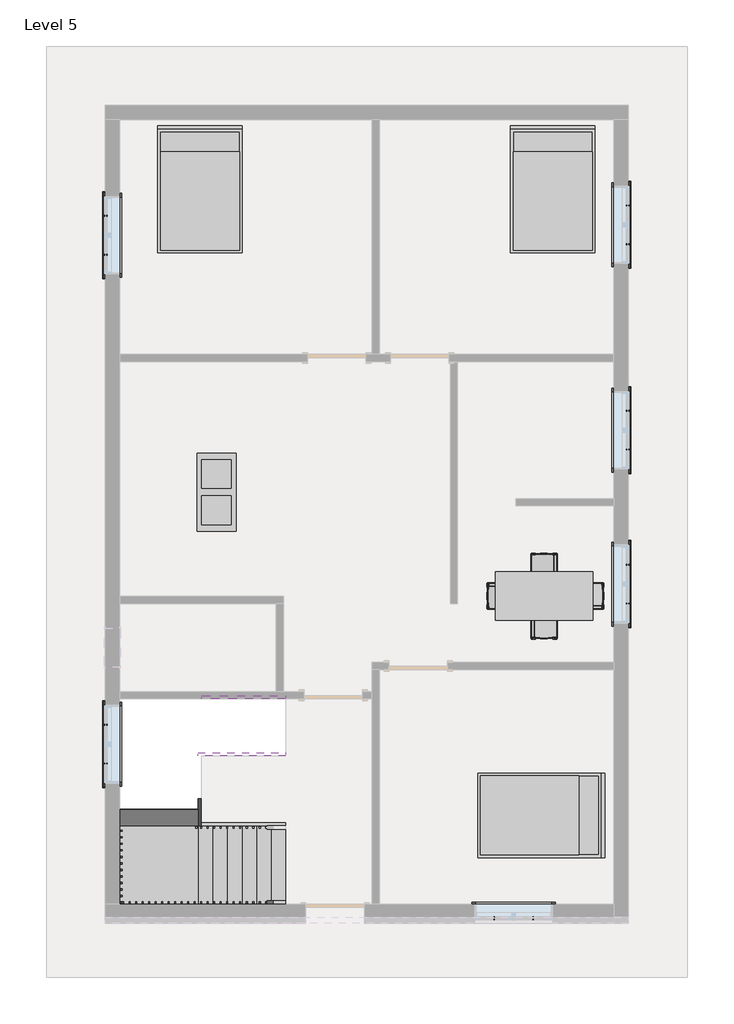
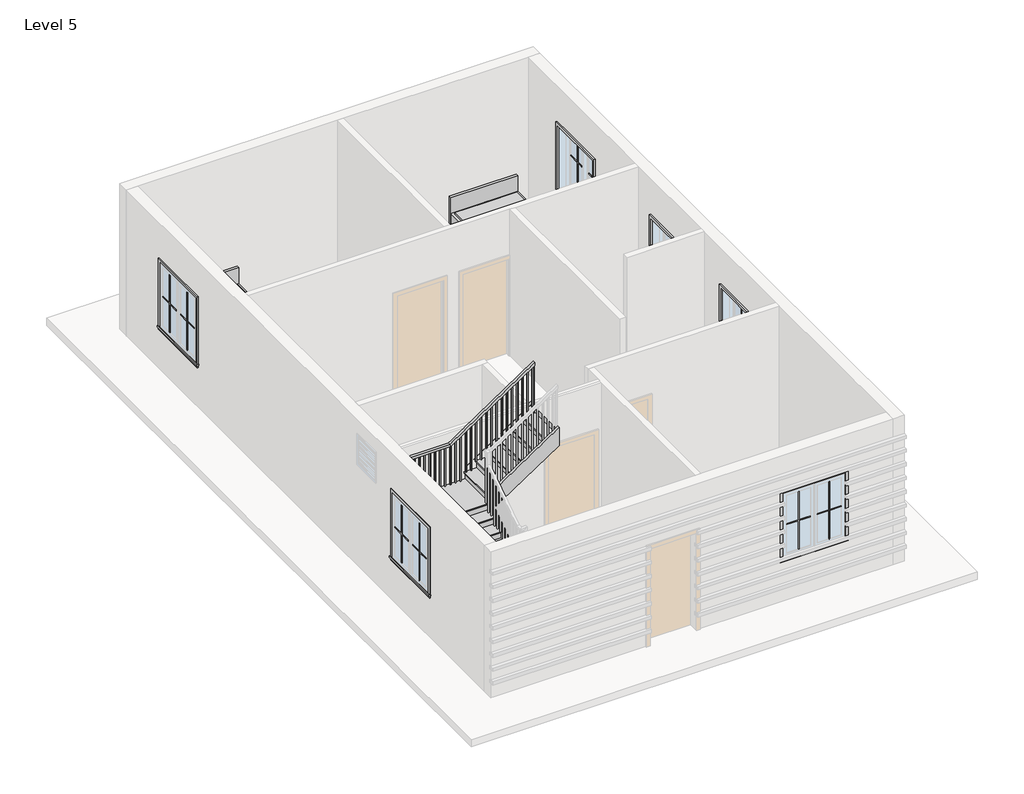
# One storey, part 3 of 3: 25 proxies, 5 members, 4 furniture elements, 1 railing, 1 stair flight.
"""IFC4 building model written with IfcOpenShell, lengths in millimetres."""

from ifc_helpers import new_model, si_unit, frame, origin, place, context, project, spatial, polyline, outline, extrude, faceted_brep, transform, mapped, element, save
from components import muntin_pattern_2x2_muntin_pattern_2x2_ba8901dc, muntin_pattern_2x2_muntin_pattern_2x2_877df4e9, trim_window_exterior_flat_with_sill_fda35bc9, trim_window_interior_flat_picture_frame_a80dbcd9, coffee_table_with_brass_mullions_11320_coffee_table_with_5962bef7, bed_17739_bed_17739_15c61121, dining_table_w_chairs_11374_0cdfc61b, stair_flight_e1114729

model = new_model("IFC4")

# Units and contexts
model_context = context("Model", 3, world=origin())
ifc_project = project(units=[si_unit("LENGTHUNIT", "METRE", prefix="MILLI")], contexts=[model_context])

# Site, building, storey
site = spatial("IfcSite", under=ifc_project)
building = spatial("IfcBuilding", under=site)
storey = spatial("IfcBuildingStorey", under=building, Name="Level 5", Elevation=12649.2)

# Proxies
placement = place(None, origin())
muntin_pattern_2x2_muntin_pattern_2x2_shape = muntin_pattern_2x2_muntin_pattern_2x2_ba8901dc(model_context)
element("IfcBuildingElementProxy", 1, Name="Muntin Pattern_2x2 : Muntin Pattern_2x2", ObjectType="Muntin Pattern_2x2 : Muntin Pattern_2x2", at=placement, inside=storey, context=model_context, shape_type="MappedRepresentation", body=[
    mapped(muntin_pattern_2x2_muntin_pattern_2x2_shape, transform((-5325.0867403, -4189.9051559, 13633.45), x_axis=(0.0, 1.0, 0.0), y_axis=(-1.0, 0.0, 0.0), z_axis=(0.0, 0.0, 1.0))),
])
element("IfcBuildingElementProxy", 2, Name="Muntin Pattern_2x2 : Muntin Pattern_2x2", ObjectType="Muntin Pattern_2x2 : Muntin Pattern_2x2", at=placement, inside=storey, context=model_context, shape_type="MappedRepresentation", body=[
    mapped(muntin_pattern_2x2_muntin_pattern_2x2_shape, transform((-5325.0867403, 3744.4198441, 13633.45), x_axis=(0.0, 1.0, 0.0), y_axis=(-1.0, 0.0, 0.0), z_axis=(0.0, 0.0, 1.0))),
])
element("IfcBuildingElementProxy", 3, Name="Muntin Pattern_2x2 : Muntin Pattern_2x2", ObjectType="Muntin Pattern_2x2 : Muntin Pattern_2x2", at=placement, inside=storey, context=model_context, shape_type="MappedRepresentation", body=[
    mapped(muntin_pattern_2x2_muntin_pattern_2x2_shape, transform((2821.9632597, 4512.7698441, 13633.45), x_axis=(0.0, -1.0, 0.0), y_axis=(1.0, 0.0, 0.0), z_axis=(0.0, 0.0, 1.0))),
])
element("IfcBuildingElementProxy", 4, Name="Muntin Pattern_2x2 : Muntin Pattern_2x2", ObjectType="Muntin Pattern_2x2 : Muntin Pattern_2x2", at=placement, inside=storey, context=model_context, shape_type="MappedRepresentation", body=[
    mapped(muntin_pattern_2x2_muntin_pattern_2x2_shape, transform((2821.9632597, 1312.3698441, 13633.45), x_axis=(0.0, -1.0, 0.0), y_axis=(1.0, 0.0, 0.0), z_axis=(0.0, 0.0, 1.0))),
])
element("IfcBuildingElementProxy", 5, Name="Muntin Pattern_2x2 : Muntin Pattern_2x2", ObjectType="Muntin Pattern_2x2 : Muntin Pattern_2x2", at=placement, inside=storey, context=model_context, shape_type="MappedRepresentation", body=[
    mapped(muntin_pattern_2x2_muntin_pattern_2x2_shape, transform((2821.9632597, -1087.9301559, 13633.45), x_axis=(0.0, -1.0, 0.0), y_axis=(1.0, 0.0, 0.0), z_axis=(0.0, 0.0, 1.0))),
])
element("IfcBuildingElementProxy", 6, Name="Muntin Pattern_2x2 : Muntin Pattern_2x2", ObjectType="Muntin Pattern_2x2 : Muntin Pattern_2x2", at=placement, inside=storey, context=model_context, shape_type="MappedRepresentation", body=[
    mapped(muntin_pattern_2x2_muntin_pattern_2x2_shape, transform((1344.0007597, -6601.3176559, 13633.45), x_axis=(-1.0, 0.0, 0.0), y_axis=(0.0, -1.0, 0.0), z_axis=(0.0, 0.0, 1.0))),
])
muntin_pattern_2x2_muntin_pattern_2x2_2_shape = muntin_pattern_2x2_muntin_pattern_2x2_877df4e9(model_context)
element("IfcBuildingElementProxy", 7, Name="Muntin Pattern_2x2 : Muntin Pattern_2x2", ObjectType="Muntin Pattern_2x2 : Muntin Pattern_2x2", at=placement, inside=storey, context=model_context, shape_type="MappedRepresentation", body=[
    mapped(muntin_pattern_2x2_muntin_pattern_2x2_2_shape, transform((-5325.0867403, -3583.4801559, 13633.45), x_axis=(0.0, -1.0, 0.0), y_axis=(1.0, 0.0, 0.0), z_axis=(0.0, 0.0, 1.0))),
])
element("IfcBuildingElementProxy", 8, Name="Muntin Pattern_2x2 : Muntin Pattern_2x2", ObjectType="Muntin Pattern_2x2 : Muntin Pattern_2x2", at=placement, inside=storey, context=model_context, shape_type="MappedRepresentation", body=[
    mapped(muntin_pattern_2x2_muntin_pattern_2x2_2_shape, transform((-5325.0867403, 4350.8448441, 13633.45), x_axis=(0.0, -1.0, 0.0), y_axis=(1.0, 0.0, 0.0), z_axis=(0.0, 0.0, 1.0))),
])
element("IfcBuildingElementProxy", 9, Name="Muntin Pattern_2x2 : Muntin Pattern_2x2", ObjectType="Muntin Pattern_2x2 : Muntin Pattern_2x2", at=placement, inside=storey, context=model_context, shape_type="MappedRepresentation", body=[
    mapped(muntin_pattern_2x2_muntin_pattern_2x2_2_shape, transform((2821.9632597, 3906.3448441, 13633.45), x_axis=(0.0, 1.0, 0.0), y_axis=(-1.0, 0.0, 0.0), z_axis=(0.0, 0.0, 1.0))),
])
element("IfcBuildingElementProxy", 10, Name="Muntin Pattern_2x2 : Muntin Pattern_2x2", ObjectType="Muntin Pattern_2x2 : Muntin Pattern_2x2", at=placement, inside=storey, context=model_context, shape_type="MappedRepresentation", body=[
    mapped(muntin_pattern_2x2_muntin_pattern_2x2_2_shape, transform((2821.9632597, 705.9448441, 13633.45), x_axis=(0.0, 1.0, 0.0), y_axis=(-1.0, 0.0, 0.0), z_axis=(0.0, 0.0, 1.0))),
])
element("IfcBuildingElementProxy", 11, Name="Muntin Pattern_2x2 : Muntin Pattern_2x2", ObjectType="Muntin Pattern_2x2 : Muntin Pattern_2x2", at=placement, inside=storey, context=model_context, shape_type="MappedRepresentation", body=[
    mapped(muntin_pattern_2x2_muntin_pattern_2x2_2_shape, transform((2821.9632597, -1694.3551559, 13633.45), x_axis=(0.0, 1.0, 0.0), y_axis=(-1.0, 0.0, 0.0), z_axis=(0.0, 0.0, 1.0))),
])
element("IfcBuildingElementProxy", 12, Name="Muntin Pattern_2x2 : Muntin Pattern_2x2", ObjectType="Muntin Pattern_2x2 : Muntin Pattern_2x2", at=placement, inside=storey, context=model_context, shape_type="MappedRepresentation", body=[
    mapped(muntin_pattern_2x2_muntin_pattern_2x2_2_shape, transform((737.5757597, -6601.3176559, 13633.45), x_axis=(1.0, 0.0, 0.0), y_axis=(0.0, 1.0, 0.0), z_axis=(0.0, 0.0, 1.0))),
])
trim_window_exterior_flat_with_sill_shape = trim_window_exterior_flat_with_sill_fda35bc9(model_context)
element("IfcBuildingElementProxy", 13, Name="Trim-Window-Exterior-Flat : with Sill", ObjectType="Trim-Window-Exterior-Flat : with Sill", at=placement, inside=storey, context=model_context, shape_type="MappedRepresentation", body=[
    mapped(trim_window_exterior_flat_with_sill_shape, transform((-5334.6117403, -3886.6926559, 14909.8), x_axis=(0.0, -1.0, 0.0), y_axis=(0.0, 0.0, 1.0), z_axis=(-1.0, 0.0, 0.0))),
])
element("IfcBuildingElementProxy", 14, Name="Trim-Window-Exterior-Flat : with Sill", ObjectType="Trim-Window-Exterior-Flat : with Sill", at=placement, inside=storey, context=model_context, shape_type="MappedRepresentation", body=[
    mapped(trim_window_exterior_flat_with_sill_shape, transform((-5334.6117403, 4047.6323441, 14909.8), x_axis=(0.0, -1.0, 0.0), y_axis=(0.0, 0.0, 1.0), z_axis=(-1.0, 0.0, 0.0))),
])
element("IfcBuildingElementProxy", 15, Name="Trim-Window-Exterior-Flat : with Sill", ObjectType="Trim-Window-Exterior-Flat : with Sill", at=placement, inside=storey, context=model_context, shape_type="MappedRepresentation", body=[
    mapped(trim_window_exterior_flat_with_sill_shape, transform((2831.4882597, 4209.5573441, 14909.8), x_axis=(0.0, 1.0, 0.0), y_axis=(0.0, 0.0, 1.0), z_axis=(1.0, 0.0, 0.0))),
])
element("IfcBuildingElementProxy", 16, Name="Trim-Window-Exterior-Flat : with Sill", ObjectType="Trim-Window-Exterior-Flat : with Sill", at=placement, inside=storey, context=model_context, shape_type="MappedRepresentation", body=[
    mapped(trim_window_exterior_flat_with_sill_shape, transform((2831.4882597, 1009.1573441, 14909.8), x_axis=(0.0, 1.0, 0.0), y_axis=(0.0, 0.0, 1.0), z_axis=(1.0, 0.0, 0.0))),
])
element("IfcBuildingElementProxy", 17, Name="Trim-Window-Exterior-Flat : with Sill", ObjectType="Trim-Window-Exterior-Flat : with Sill", at=placement, inside=storey, context=model_context, shape_type="MappedRepresentation", body=[
    mapped(trim_window_exterior_flat_with_sill_shape, transform((2831.4882597, -1391.1426559, 14909.8), x_axis=(0.0, 1.0, 0.0), y_axis=(0.0, 0.0, 1.0), z_axis=(1.0, 0.0, 0.0))),
])
element("IfcBuildingElementProxy", 18, Name="Trim-Window-Exterior-Flat : with Sill", ObjectType="Trim-Window-Exterior-Flat : with Sill", at=placement, inside=storey, context=model_context, shape_type="MappedRepresentation", body=[
    mapped(trim_window_exterior_flat_with_sill_shape, transform((1040.7882597, -6610.8426559, 14909.8), x_axis=(1.0, 0.0, 0.0), y_axis=(0.0, 0.0, 1.0), z_axis=(0.0, -1.0, 0.0))),
])
trim_window_interior_flat_picture_frame_shape = trim_window_interior_flat_picture_frame_a80dbcd9(model_context)
element("IfcBuildingElementProxy", 19, Name="Trim-Window-Interior-Flat : Picture Frame", ObjectType="Trim-Window-Interior-Flat : Picture Frame", at=placement, inside=storey, context=model_context, shape_type="MappedRepresentation", body=[
    mapped(trim_window_interior_flat_picture_frame_shape, transform((-5106.0117403, -3886.6926559, 14909.8), x_axis=(0.0, 1.0, 0.0), y_axis=(0.0, 0.0, 1.0), z_axis=(1.0, 0.0, 0.0))),
])
element("IfcBuildingElementProxy", 20, Name="Trim-Window-Interior-Flat : Picture Frame", ObjectType="Trim-Window-Interior-Flat : Picture Frame", at=placement, inside=storey, context=model_context, shape_type="MappedRepresentation", body=[
    mapped(trim_window_interior_flat_picture_frame_shape, transform((-5106.0117403, 4047.6323441, 14909.8), x_axis=(0.0, 1.0, 0.0), y_axis=(0.0, 0.0, 1.0), z_axis=(1.0, 0.0, 0.0))),
])
element("IfcBuildingElementProxy", 21, Name="Trim-Window-Interior-Flat : Picture Frame", ObjectType="Trim-Window-Interior-Flat : Picture Frame", at=placement, inside=storey, context=model_context, shape_type="MappedRepresentation", body=[
    mapped(trim_window_interior_flat_picture_frame_shape, transform((2602.8882597, 4209.5573441, 14909.8), x_axis=(0.0, -1.0, 0.0), y_axis=(0.0, 0.0, 1.0), z_axis=(-1.0, 0.0, 0.0))),
])
element("IfcBuildingElementProxy", 22, Name="Trim-Window-Interior-Flat : Picture Frame", ObjectType="Trim-Window-Interior-Flat : Picture Frame", at=placement, inside=storey, context=model_context, shape_type="MappedRepresentation", body=[
    mapped(trim_window_interior_flat_picture_frame_shape, transform((2602.8882597, 1009.1573441, 14909.8), x_axis=(0.0, -1.0, 0.0), y_axis=(0.0, 0.0, 1.0), z_axis=(-1.0, 0.0, 0.0))),
])
element("IfcBuildingElementProxy", 23, Name="Trim-Window-Interior-Flat : Picture Frame", ObjectType="Trim-Window-Interior-Flat : Picture Frame", at=placement, inside=storey, context=model_context, shape_type="MappedRepresentation", body=[
    mapped(trim_window_interior_flat_picture_frame_shape, transform((2602.8882597, -1391.1426559, 14909.8), x_axis=(0.0, -1.0, 0.0), y_axis=(0.0, 0.0, 1.0), z_axis=(-1.0, 0.0, 0.0))),
])
element("IfcBuildingElementProxy", 24, Name="Trim-Window-Interior-Flat : Picture Frame", ObjectType="Trim-Window-Interior-Flat : Picture Frame", at=placement, inside=storey, context=model_context, shape_type="MappedRepresentation", body=[
    mapped(trim_window_interior_flat_picture_frame_shape, transform((1040.7882597, -6382.2426559, 14909.8), x_axis=(-1.0, 0.0, 0.0), y_axis=(0.0, 0.0, 1.0), z_axis=(0.0, 1.0, 0.0))),
])
coffee_table_with_brass_mullions_11320_coffee_table_with_shape = coffee_table_with_brass_mullions_11320_coffee_table_with_5962bef7(model_context)
element("IfcBuildingElementProxy", 25, Name="coffee_table_with_brass_mullions_11320 : coffee_table_with_brass_mullions_11320", ObjectType="coffee_table_with_brass_mullions_11320 : coffee_table_with_brass_mullions_11320", at=placement, inside=storey, context=model_context, shape_type="MappedRepresentation", body=[
    mapped(coffee_table_with_brass_mullions_11320_coffee_table_with_shape, transform((-3162.9117403, 678.9573441, 12649.2), x_axis=(0.0, 1.0, 0.0), y_axis=(-1.0, 0.0, 0.0), z_axis=(0.0, 0.0, 1.0))),
])

# Furniture
bed_17739_bed_17739_shape = bed_17739_bed_17739_15c61121(model_context)
element("IfcFurniture", 26, ObjectType="Bed_17739 : Bed_17739", at=placement, inside=storey, context=model_context, shape_type="MappedRepresentation", body=[
    mapped(bed_17739_bed_17739_shape, transform((-3855.0617403, 4742.9573441, 12649.2), x_axis=(1.0, 0.0, 0.0), y_axis=(0.0, 1.0, 0.0), z_axis=(0.0, 0.0, 1.0))),
])
element("IfcFurniture", 27, ObjectType="Bed_17739 : Bed_17739", at=placement, inside=storey, context=model_context, shape_type="MappedRepresentation", body=[
    mapped(bed_17739_bed_17739_shape, transform((1650.3882597, 4742.9573441, 12649.2), x_axis=(1.0, 0.0, 0.0), y_axis=(0.0, 1.0, 0.0), z_axis=(0.0, 0.0, 1.0))),
])
element("IfcFurniture", 28, ObjectType="Bed_17739 : Bed_17739", at=placement, inside=storey, context=model_context, shape_type="MappedRepresentation", body=[
    mapped(bed_17739_bed_17739_shape, transform((1447.1882597, -4997.9426559, 12649.2), x_axis=(0.0, -1.0, 0.0), y_axis=(1.0, 0.0, 0.0), z_axis=(0.0, 0.0, 1.0))),
])
dining_table_w_chairs_11374_shape = dining_table_w_chairs_11374_0cdfc61b(model_context)
element("IfcFurniture", 29, ObjectType="Dining_Table_w_Chairs_11374", at=placement, inside=storey, context=model_context, shape_type="MappedRepresentation", body=[
    mapped(dining_table_w_chairs_11374_shape, transform((1497.0410232, -1671.6886654, 12649.2), x_axis=(1.0, 0.0, 0.0), y_axis=(0.0, 1.0, 0.0), z_axis=(0.0, 0.0, 1.0))),
])

# Members
element("IfcMember", 30, ObjectType="Stringer - 2\" Width", at=placement, inside=storey, context=model_context, shape_type="SweptSolid", body=[
    extrude(outline(polyline([(12649.2, -2515.2117403), (12867.2398409, -2515.2117403), (13121.2398409, -2896.2117403), (13121.2398409, -3445.6977546), (12649.2, -2737.6379933), (12649.2, -2515.2117403)])), frame((0.0, -6433.0426559, 0.0), z_axis=(0.0, 1.0, 0.0), x_axis=(0.0, 0.0, 1.0)), (0.0, 0.0, 1.0), 50.8),
])
element("IfcMember", 31, ObjectType="Stringer - 2\" Width", at=placement, inside=storey, context=model_context, shape_type="SweptSolid", body=[
    extrude(outline(polyline([(14888.5158313, -3277.2117403), (15396.5158313, -2515.2117403), (15762.8398409, -2515.2117403), (14888.5158313, -3826.6977546), (14888.5158313, -3277.2117403)])), frame((0.0, -3181.8426559, 0.0), z_axis=(0.0, 1.0, 0.0), x_axis=(0.0, 0.0, 1.0)), (0.0, 0.0, 1.0), 50.8),
])
element("IfcMember", 32, ObjectType="Stringer - 2\" Width", at=placement, inside=storey, context=model_context, shape_type="SweptSolid", body=[
    extrude(outline(polyline([(12649.2, -2515.2117403), (12867.2398409, -2515.2117403), (13747.7731743, -3836.0117403), (13381.4491647, -3836.0117403), (12649.2, -2737.6379933), (12649.2, -2515.2117403)])), frame((0.0, -5163.0426559, 0.0), z_axis=(0.0, 1.0, 0.0), x_axis=(0.0, 0.0, 1.0)), (0.0, 0.0, 1.0), 50.8),
])
element("IfcMember", 33, ObjectType="Stringer - 2\" Width", at=placement, inside=storey, context=model_context, shape_type="SweptSolid", body=[
    extrude(outline(polyline([(-5163.0426559, 13567.7158313), (-5163.0426559, 13934.0398409), (-4070.8426559, 14662.1731743), (-4070.8426559, 14295.8491647), (-5163.0426559, 13567.7158313)])), frame((-3886.8117403, 0.0, 0.0), z_axis=(1.0, 0.0, 0.0), x_axis=(0.0, 1.0, 0.0)), (0.0, 0.0, 1.0), 50.8),
])
element("IfcMember", 34, ObjectType="Stringer - 2\" Width", at=placement, inside=storey, context=model_context, shape_type="SweptSolid", body=[
    extrude(outline(polyline([(14848.4398409, -3886.8117403), (14482.1158313, -3886.8117403), (15396.5158313, -2515.2117403), (15762.8398409, -2515.2117403), (14848.4398409, -3886.8117403)])), frame((0.0, -4070.8426559, 0.0), z_axis=(0.0, 1.0, 0.0), x_axis=(0.0, 0.0, 1.0)), (0.0, 0.0, 1.0), 50.8),
])

# Railing
element("IfcRailing", 35, ObjectType="Handrail - Rectangular", at=placement, inside=storey, context=model_context, shape_type="SolidModel", body=[
    faceted_brep([(-2515.2117403, -6382.2426559, 13716.0), (-2515.2117403, -6382.2426559, 13654.9459984), (-2515.2117403, -6331.4426559, 13654.9459984), (-2515.2117403, -6331.4426559, 13716.0), (-4001.1117403, -6382.2426559, 14706.6), (-4016.4927427, -6382.2426559, 14655.8), (-4016.4927427, -6331.4426559, 14655.8), (-4001.1117403, -6331.4426559, 14706.6), (-5106.0117403, -6382.2426559, 14706.6), (-5106.0117403, -6382.2426559, 14655.8), (-5055.2117403, -6331.4426559, 14655.8), (-5055.2117403, -6331.4426559, 14706.6), (-5106.0117403, -5277.3426559, 14706.6), (-5106.0117403, -5261.9616535, 14655.8), (-5055.2117403, -5261.9616535, 14655.8), (-5055.2117403, -5277.3426559, 14706.6), (-5106.0117403, -4096.2426559, 15494.0), (-5106.0117403, -4080.8616535, 15443.2), (-5055.2117403, -4080.8616535, 15443.2), (-5055.2117403, -4096.2426559, 15494.0), (-5106.0117403, -3181.8426559, 15494.0), (-5106.0117403, -3181.8426559, 15443.2), (-5055.2117403, -3232.6426559, 15443.2), (-5055.2117403, -3232.6426559, 15494.0), (-4191.6117403, -3181.8426559, 15494.0), (-4176.2307379, -3181.8426559, 15443.2), (-4176.2307379, -3232.6426559, 15443.2), (-4191.6117403, -3232.6426559, 15494.0), (-2515.2117403, -3181.8426559, 16611.6), (-2515.2117403, -3232.6426559, 16611.6), (-2515.2117403, -3232.6426559, 16550.5459984), (-2515.2117403, -3181.8426559, 16550.5459984)], [[[0, 1, 2, 3]], [[1, 0, 4, 5]], [[2, 1, 5, 6]], [[3, 2, 6, 7]], [[0, 3, 7, 4]], [[5, 4, 8, 9]], [[6, 5, 9, 10]], [[7, 6, 10, 11]], [[4, 7, 11, 8]], [[9, 8, 12, 13]], [[10, 9, 13, 14]], [[11, 10, 14, 15]], [[8, 11, 15, 12]], [[13, 12, 16, 17]], [[14, 13, 17, 18]], [[15, 14, 18, 19]], [[12, 15, 19, 16]], [[17, 16, 20, 21]], [[18, 17, 21, 22]], [[19, 18, 22, 23]], [[16, 19, 23, 20]], [[21, 20, 24, 25]], [[22, 21, 25, 26]], [[23, 22, 26, 27]], [[20, 23, 27, 24]], [[28, 29, 30, 31]], [[25, 24, 28, 31]], [[26, 25, 31, 30]], [[27, 26, 30, 29]], [[24, 27, 29, 28]]]),
    extrude(outline(polyline([(16527.2626651, -2550.1367403), (15544.8, -2550.1367403), (15544.8, -2531.0867403), (16539.9626651, -2531.0867403), (16527.2626651, -2550.1367403)])), frame((0.0, -3216.7676559, 0.0), z_axis=(0.0, 1.0, 0.0), x_axis=(0.0, 0.0, 1.0)), (0.0, 0.0, 1.0), 19.05),
    extrude(outline(polyline([(16459.5293317, -2651.7367403), (15544.8, -2651.7367403), (15544.8, -2632.6867403), (16472.2293317, -2632.6867403), (16459.5293317, -2651.7367403)])), frame((0.0, -3216.7676559, 0.0), z_axis=(0.0, 1.0, 0.0), x_axis=(0.0, 0.0, 1.0)), (0.0, 0.0, 1.0), 19.05),
    extrude(outline(polyline([(16391.7959984, -2753.3367403), (15544.8, -2753.3367403), (15544.8, -2734.2867403), (16404.4959984, -2734.2867403), (16391.7959984, -2753.3367403)])), frame((0.0, -3216.7676559, 0.0), z_axis=(0.0, 1.0, 0.0), x_axis=(0.0, 0.0, 1.0)), (0.0, 0.0, 1.0), 19.05),
    extrude(outline(polyline([(16324.0626651, -2854.9367403), (15392.4, -2854.9367403), (15392.4, -2835.8867403), (16336.7626651, -2835.8867403), (16324.0626651, -2854.9367403)])), frame((0.0, -3216.7676559, 0.0), z_axis=(0.0, 1.0, 0.0), x_axis=(0.0, 0.0, 1.0)), (0.0, 0.0, 1.0), 19.05),
    extrude(outline(polyline([(16256.3293317, -2956.5367403), (15392.4, -2956.5367403), (15392.4, -2937.4867403), (16269.0293317, -2937.4867403), (16256.3293317, -2956.5367403)])), frame((0.0, -3216.7676559, 0.0), z_axis=(0.0, 1.0, 0.0), x_axis=(0.0, 0.0, 1.0)), (0.0, 0.0, 1.0), 19.05),
    extrude(outline(polyline([(16188.5959984, -3058.1367403), (15240.0, -3058.1367403), (15240.0, -3039.0867403), (16201.2959984, -3039.0867403), (16188.5959984, -3058.1367403)])), frame((0.0, -3216.7676559, 0.0), z_axis=(0.0, 1.0, 0.0), x_axis=(0.0, 0.0, 1.0)), (0.0, 0.0, 1.0), 19.05),
    extrude(outline(polyline([(16120.8626651, -3159.7367403), (15240.0, -3159.7367403), (15240.0, -3140.6867403), (16133.5626651, -3140.6867403), (16120.8626651, -3159.7367403)])), frame((0.0, -3216.7676559, 0.0), z_axis=(0.0, 1.0, 0.0), x_axis=(0.0, 0.0, 1.0)), (0.0, 0.0, 1.0), 19.05),
    extrude(outline(polyline([(16053.1293317, -3261.3367403), (15087.6, -3261.3367403), (15087.6, -3242.2867403), (16065.8293317, -3242.2867403), (16053.1293317, -3261.3367403)])), frame((0.0, -3216.7676559, 0.0), z_axis=(0.0, 1.0, 0.0), x_axis=(0.0, 0.0, 1.0)), (0.0, 0.0, 1.0), 19.05),
    extrude(outline(polyline([(15985.3959984, -3362.9367403), (15087.6, -3362.9367403), (15087.6, -3343.8867403), (15998.0959984, -3343.8867403), (15985.3959984, -3362.9367403)])), frame((0.0, -3216.7676559, 0.0), z_axis=(0.0, 1.0, 0.0), x_axis=(0.0, 0.0, 1.0)), (0.0, 0.0, 1.0), 19.05),
    extrude(outline(polyline([(15917.6626651, -3464.5367403), (14935.2, -3464.5367403), (14935.2, -3445.4867403), (15930.3626651, -3445.4867403), (15917.6626651, -3464.5367403)])), frame((0.0, -3216.7676559, 0.0), z_axis=(0.0, 1.0, 0.0), x_axis=(0.0, 0.0, 1.0)), (0.0, 0.0, 1.0), 19.05),
    extrude(outline(polyline([(15849.9293317, -3566.1367403), (14935.2, -3566.1367403), (14935.2, -3547.0867403), (15862.6293317, -3547.0867403), (15849.9293317, -3566.1367403)])), frame((0.0, -3216.7676559, 0.0), z_axis=(0.0, 1.0, 0.0), x_axis=(0.0, 0.0, 1.0)), (0.0, 0.0, 1.0), 19.05),
    extrude(outline(polyline([(15782.1959984, -3667.7367403), (14935.2, -3667.7367403), (14935.2, -3648.6867403), (15794.8959984, -3648.6867403), (15782.1959984, -3667.7367403)])), frame((0.0, -3216.7676559, 0.0), z_axis=(0.0, 1.0, 0.0), x_axis=(0.0, 0.0, 1.0)), (0.0, 0.0, 1.0), 19.05),
    extrude(outline(polyline([(15714.4626651, -3769.3367403), (14782.8, -3769.3367403), (14782.8, -3750.2867403), (15727.1626651, -3750.2867403), (15714.4626651, -3769.3367403)])), frame((0.0, -3216.7676559, 0.0), z_axis=(0.0, 1.0, 0.0), x_axis=(0.0, 0.0, 1.0)), (0.0, 0.0, 1.0), 19.05),
    extrude(outline(polyline([(15646.7293317, -3870.9367403), (14782.8, -3870.9367403), (14782.8, -3851.8867403), (15659.4293317, -3851.8867403), (15646.7293317, -3870.9367403)])), frame((0.0, -3216.7676559, 0.0), z_axis=(0.0, 1.0, 0.0), x_axis=(0.0, 0.0, 1.0)), (0.0, 0.0, 1.0), 19.05),
    extrude(outline(polyline([(15578.9959984, -3972.5367403), (14630.4, -3972.5367403), (14630.4, -3953.4867403), (15591.6959984, -3953.4867403), (15578.9959984, -3972.5367403)])), frame((0.0, -3216.7676559, 0.0), z_axis=(0.0, 1.0, 0.0), x_axis=(0.0, 0.0, 1.0)), (0.0, 0.0, 1.0), 19.05),
    extrude(outline(polyline([(15511.2626651, -4074.1367403), (14630.4, -4074.1367403), (14630.4, -4055.0867403), (15523.9626651, -4055.0867403), (15511.2626651, -4074.1367403)])), frame((0.0, -3216.7676559, 0.0), z_axis=(0.0, 1.0, 0.0), x_axis=(0.0, 0.0, 1.0)), (0.0, 0.0, 1.0), 19.05),
    extrude(outline(polyline([(15443.5293317, -4175.7367403), (14630.4, -4175.7367403), (14630.4, -4156.6867403), (15456.2293317, -4156.6867403), (15443.5293317, -4175.7367403)])), frame((0.0, -3216.7676559, 0.0), z_axis=(0.0, 1.0, 0.0), x_axis=(0.0, 0.0, 1.0)), (0.0, 0.0, 1.0), 19.05),
    extrude(outline(polyline([(-4277.3367403, -3197.7176559), (-4258.2867403, -3197.7176559), (-4258.2867403, -3216.7676559), (-4277.3367403, -3216.7676559), (-4277.3367403, -3197.7176559)])), frame((0.0, 0.0, 14630.4), z_axis=(0.0, 0.0, 1.0), x_axis=(1.0, 0.0, 0.0)), (0.0, 0.0, 1.0), 812.8),
    extrude(outline(polyline([(-4378.9367403, -3197.7176559), (-4359.8867403, -3197.7176559), (-4359.8867403, -3216.7676559), (-4378.9367403, -3216.7676559), (-4378.9367403, -3197.7176559)])), frame((0.0, 0.0, 14630.4), z_axis=(0.0, 0.0, 1.0), x_axis=(1.0, 0.0, 0.0)), (0.0, 0.0, 1.0), 812.8),
    extrude(outline(polyline([(-4480.5367403, -3197.7176559), (-4461.4867403, -3197.7176559), (-4461.4867403, -3216.7676559), (-4480.5367403, -3216.7676559), (-4480.5367403, -3197.7176559)])), frame((0.0, 0.0, 14630.4), z_axis=(0.0, 0.0, 1.0), x_axis=(1.0, 0.0, 0.0)), (0.0, 0.0, 1.0), 812.8),
    extrude(outline(polyline([(-4582.1367403, -3197.7176559), (-4563.0867403, -3197.7176559), (-4563.0867403, -3216.7676559), (-4582.1367403, -3216.7676559), (-4582.1367403, -3197.7176559)])), frame((0.0, 0.0, 14630.4), z_axis=(0.0, 0.0, 1.0), x_axis=(1.0, 0.0, 0.0)), (0.0, 0.0, 1.0), 812.8),
    extrude(outline(polyline([(-4683.7367403, -3197.7176559), (-4664.6867403, -3197.7176559), (-4664.6867403, -3216.7676559), (-4683.7367403, -3216.7676559), (-4683.7367403, -3197.7176559)])), frame((0.0, 0.0, 14630.4), z_axis=(0.0, 0.0, 1.0), x_axis=(1.0, 0.0, 0.0)), (0.0, 0.0, 1.0), 812.8),
    extrude(outline(polyline([(-4785.3367403, -3197.7176559), (-4766.2867403, -3197.7176559), (-4766.2867403, -3216.7676559), (-4785.3367403, -3216.7676559), (-4785.3367403, -3197.7176559)])), frame((0.0, 0.0, 14630.4), z_axis=(0.0, 0.0, 1.0), x_axis=(1.0, 0.0, 0.0)), (0.0, 0.0, 1.0), 812.8),
    extrude(outline(polyline([(-4886.9367403, -3197.7176559), (-4867.8867403, -3197.7176559), (-4867.8867403, -3216.7676559), (-4886.9367403, -3216.7676559), (-4886.9367403, -3197.7176559)])), frame((0.0, 0.0, 14630.4), z_axis=(0.0, 0.0, 1.0), x_axis=(1.0, 0.0, 0.0)), (0.0, 0.0, 1.0), 812.8),
    extrude(outline(polyline([(-4988.5367403, -3197.7176559), (-4969.4867403, -3197.7176559), (-4969.4867403, -3216.7676559), (-4988.5367403, -3216.7676559), (-4988.5367403, -3197.7176559)])), frame((0.0, 0.0, 14630.4), z_axis=(0.0, 0.0, 1.0), x_axis=(1.0, 0.0, 0.0)), (0.0, 0.0, 1.0), 812.8),
    extrude(outline(polyline([(-5090.1367403, -3318.3676559), (-5090.1367403, -3299.3176559), (-5071.0867403, -3299.3176559), (-5071.0867403, -3318.3676559), (-5090.1367403, -3318.3676559)])), frame((0.0, 0.0, 14630.4), z_axis=(0.0, 0.0, 1.0), x_axis=(1.0, 0.0, 0.0)), (0.0, 0.0, 1.0), 812.8),
    extrude(outline(polyline([(-5090.1367403, -3419.9676559), (-5090.1367403, -3400.9176559), (-5071.0867403, -3400.9176559), (-5071.0867403, -3419.9676559), (-5090.1367403, -3419.9676559)])), frame((0.0, 0.0, 14630.4), z_axis=(0.0, 0.0, 1.0), x_axis=(1.0, 0.0, 0.0)), (0.0, 0.0, 1.0), 812.8),
    extrude(outline(polyline([(-5090.1367403, -3521.5676559), (-5090.1367403, -3502.5176559), (-5071.0867403, -3502.5176559), (-5071.0867403, -3521.5676559), (-5090.1367403, -3521.5676559)])), frame((0.0, 0.0, 14630.4), z_axis=(0.0, 0.0, 1.0), x_axis=(1.0, 0.0, 0.0)), (0.0, 0.0, 1.0), 812.8),
    extrude(outline(polyline([(-5090.1367403, -3623.1676559), (-5090.1367403, -3604.1176559), (-5071.0867403, -3604.1176559), (-5071.0867403, -3623.1676559), (-5090.1367403, -3623.1676559)])), frame((0.0, 0.0, 14630.4), z_axis=(0.0, 0.0, 1.0), x_axis=(1.0, 0.0, 0.0)), (0.0, 0.0, 1.0), 812.8),
    extrude(outline(polyline([(-5090.1367403, -3724.7676559), (-5090.1367403, -3705.7176559), (-5071.0867403, -3705.7176559), (-5071.0867403, -3724.7676559), (-5090.1367403, -3724.7676559)])), frame((0.0, 0.0, 14630.4), z_axis=(0.0, 0.0, 1.0), x_axis=(1.0, 0.0, 0.0)), (0.0, 0.0, 1.0), 812.8),
    extrude(outline(polyline([(-5090.1367403, -3826.3676559), (-5090.1367403, -3807.3176559), (-5071.0867403, -3807.3176559), (-5071.0867403, -3826.3676559), (-5090.1367403, -3826.3676559)])), frame((0.0, 0.0, 14630.4), z_axis=(0.0, 0.0, 1.0), x_axis=(1.0, 0.0, 0.0)), (0.0, 0.0, 1.0), 812.8),
    extrude(outline(polyline([(-5090.1367403, -3927.9676559), (-5090.1367403, -3908.9176559), (-5071.0867403, -3908.9176559), (-5071.0867403, -3927.9676559), (-5090.1367403, -3927.9676559)])), frame((0.0, 0.0, 14630.4), z_axis=(0.0, 0.0, 1.0), x_axis=(1.0, 0.0, 0.0)), (0.0, 0.0, 1.0), 812.8),
    extrude(outline(polyline([(-5090.1367403, -4029.5676559), (-5090.1367403, -4010.5176559), (-5071.0867403, -4010.5176559), (-5071.0867403, -4029.5676559), (-5090.1367403, -4029.5676559)])), frame((0.0, 0.0, 14630.4), z_axis=(0.0, 0.0, 1.0), x_axis=(1.0, 0.0, 0.0)), (0.0, 0.0, 1.0), 812.8),
    extrude(outline(polyline([(-4112.1176559, 15422.3626651), (-4112.1176559, 14478.0), (-4131.1676559, 14478.0), (-4131.1676559, 15409.6626651), (-4112.1176559, 15422.3626651)])), frame((-5090.1367403, 0.0, 0.0), z_axis=(1.0, 0.0, 0.0), x_axis=(0.0, 1.0, 0.0)), (0.0, 0.0, 1.0), 19.05),
    extrude(outline(polyline([(-4213.7176559, 15354.6293317), (-4213.7176559, 14478.0), (-4232.7676559, 14478.0), (-4232.7676559, 15341.9293317), (-4213.7176559, 15354.6293317)])), frame((-5090.1367403, 0.0, 0.0), z_axis=(1.0, 0.0, 0.0), x_axis=(0.0, 1.0, 0.0)), (0.0, 0.0, 1.0), 19.05),
    extrude(outline(polyline([(-4315.3176559, 15286.8959984), (-4315.3176559, 14325.6), (-4334.3676559, 14325.6), (-4334.3676559, 15274.1959984), (-4315.3176559, 15286.8959984)])), frame((-5090.1367403, 0.0, 0.0), z_axis=(1.0, 0.0, 0.0), x_axis=(0.0, 1.0, 0.0)), (0.0, 0.0, 1.0), 19.05),
    extrude(outline(polyline([(-4416.9176559, 15219.1626651), (-4416.9176559, 14325.6), (-4435.9676559, 14325.6), (-4435.9676559, 15206.4626651), (-4416.9176559, 15219.1626651)])), frame((-5090.1367403, 0.0, 0.0), z_axis=(1.0, 0.0, 0.0), x_axis=(0.0, 1.0, 0.0)), (0.0, 0.0, 1.0), 19.05),
    extrude(outline(polyline([(-4518.5176559, 15151.4293317), (-4518.5176559, 14173.2), (-4537.5676559, 14173.2), (-4537.5676559, 15138.7293317), (-4518.5176559, 15151.4293317)])), frame((-5090.1367403, 0.0, 0.0), z_axis=(1.0, 0.0, 0.0), x_axis=(0.0, 1.0, 0.0)), (0.0, 0.0, 1.0), 19.05),
    extrude(outline(polyline([(-4620.1176559, 15083.6959984), (-4620.1176559, 14173.2), (-4639.1676559, 14173.2), (-4639.1676559, 15070.9959984), (-4620.1176559, 15083.6959984)])), frame((-5090.1367403, 0.0, 0.0), z_axis=(1.0, 0.0, 0.0), x_axis=(0.0, 1.0, 0.0)), (0.0, 0.0, 1.0), 19.05),
    extrude(outline(polyline([(-4721.7176559, 15015.9626651), (-4721.7176559, 14020.8), (-4740.7676559, 14020.8), (-4740.7676559, 15003.2626651), (-4721.7176559, 15015.9626651)])), frame((-5090.1367403, 0.0, 0.0), z_axis=(1.0, 0.0, 0.0), x_axis=(0.0, 1.0, 0.0)), (0.0, 0.0, 1.0), 19.05),
    extrude(outline(polyline([(-4823.3176559, 14948.2293317), (-4823.3176559, 14020.8), (-4842.3676559, 14020.8), (-4842.3676559, 14935.5293317), (-4823.3176559, 14948.2293317)])), frame((-5090.1367403, 0.0, 0.0), z_axis=(1.0, 0.0, 0.0), x_axis=(0.0, 1.0, 0.0)), (0.0, 0.0, 1.0), 19.05),
    extrude(outline(polyline([(-4924.9176559, 14880.4959984), (-4924.9176559, 14020.8), (-4943.9676559, 14020.8), (-4943.9676559, 14867.7959984), (-4924.9176559, 14880.4959984)])), frame((-5090.1367403, 0.0, 0.0), z_axis=(1.0, 0.0, 0.0), x_axis=(0.0, 1.0, 0.0)), (0.0, 0.0, 1.0), 19.05),
    extrude(outline(polyline([(-5026.5176559, 14812.7626651), (-5026.5176559, 13868.4), (-5045.5676559, 13868.4), (-5045.5676559, 14800.0626651), (-5026.5176559, 14812.7626651)])), frame((-5090.1367403, 0.0, 0.0), z_axis=(1.0, 0.0, 0.0), x_axis=(0.0, 1.0, 0.0)), (0.0, 0.0, 1.0), 19.05),
    extrude(outline(polyline([(-5128.1176559, 14745.0293317), (-5128.1176559, 13868.4), (-5147.1676559, 13868.4), (-5147.1676559, 14732.3293317), (-5128.1176559, 14745.0293317)])), frame((-5090.1367403, 0.0, 0.0), z_axis=(1.0, 0.0, 0.0), x_axis=(0.0, 1.0, 0.0)), (0.0, 0.0, 1.0), 19.05),
    extrude(outline(polyline([(-5229.7176559, 14677.2959984), (-5229.7176559, 13716.0), (-5248.7676559, 13716.0), (-5248.7676559, 14664.5959984), (-5229.7176559, 14677.2959984)])), frame((-5090.1367403, 0.0, 0.0), z_axis=(1.0, 0.0, 0.0), x_axis=(0.0, 1.0, 0.0)), (0.0, 0.0, 1.0), 19.05),
    extrude(outline(polyline([(-5090.1367403, -5350.3676559), (-5090.1367403, -5331.3176559), (-5071.0867403, -5331.3176559), (-5071.0867403, -5350.3676559), (-5090.1367403, -5350.3676559)])), frame((0.0, 0.0, 13716.0), z_axis=(0.0, 0.0, 1.0), x_axis=(1.0, 0.0, 0.0)), (0.0, 0.0, 1.0), 939.8),
    extrude(outline(polyline([(-5090.1367403, -5451.9676559), (-5090.1367403, -5432.9176559), (-5071.0867403, -5432.9176559), (-5071.0867403, -5451.9676559), (-5090.1367403, -5451.9676559)])), frame((0.0, 0.0, 13716.0), z_axis=(0.0, 0.0, 1.0), x_axis=(1.0, 0.0, 0.0)), (0.0, 0.0, 1.0), 939.8),
    extrude(outline(polyline([(-5090.1367403, -5553.5676559), (-5090.1367403, -5534.5176559), (-5071.0867403, -5534.5176559), (-5071.0867403, -5553.5676559), (-5090.1367403, -5553.5676559)])), frame((0.0, 0.0, 13716.0), z_axis=(0.0, 0.0, 1.0), x_axis=(1.0, 0.0, 0.0)), (0.0, 0.0, 1.0), 939.8),
    extrude(outline(polyline([(-5090.1367403, -5655.1676559), (-5090.1367403, -5636.1176559), (-5071.0867403, -5636.1176559), (-5071.0867403, -5655.1676559), (-5090.1367403, -5655.1676559)])), frame((0.0, 0.0, 13716.0), z_axis=(0.0, 0.0, 1.0), x_axis=(1.0, 0.0, 0.0)), (0.0, 0.0, 1.0), 939.8),
    extrude(outline(polyline([(-5090.1367403, -5756.7676559), (-5090.1367403, -5737.7176559), (-5071.0867403, -5737.7176559), (-5071.0867403, -5756.7676559), (-5090.1367403, -5756.7676559)])), frame((0.0, 0.0, 13716.0), z_axis=(0.0, 0.0, 1.0), x_axis=(1.0, 0.0, 0.0)), (0.0, 0.0, 1.0), 939.8),
    extrude(outline(polyline([(-5090.1367403, -5858.3676559), (-5090.1367403, -5839.3176559), (-5071.0867403, -5839.3176559), (-5071.0867403, -5858.3676559), (-5090.1367403, -5858.3676559)])), frame((0.0, 0.0, 13716.0), z_axis=(0.0, 0.0, 1.0), x_axis=(1.0, 0.0, 0.0)), (0.0, 0.0, 1.0), 939.8),
    extrude(outline(polyline([(-5090.1367403, -5959.9676559), (-5090.1367403, -5940.9176559), (-5071.0867403, -5940.9176559), (-5071.0867403, -5959.9676559), (-5090.1367403, -5959.9676559)])), frame((0.0, 0.0, 13716.0), z_axis=(0.0, 0.0, 1.0), x_axis=(1.0, 0.0, 0.0)), (0.0, 0.0, 1.0), 939.8),
    extrude(outline(polyline([(-5090.1367403, -6061.5676559), (-5090.1367403, -6042.5176559), (-5071.0867403, -6042.5176559), (-5071.0867403, -6061.5676559), (-5090.1367403, -6061.5676559)])), frame((0.0, 0.0, 13716.0), z_axis=(0.0, 0.0, 1.0), x_axis=(1.0, 0.0, 0.0)), (0.0, 0.0, 1.0), 939.8),
    extrude(outline(polyline([(-5090.1367403, -6163.1676559), (-5090.1367403, -6144.1176559), (-5071.0867403, -6144.1176559), (-5071.0867403, -6163.1676559), (-5090.1367403, -6163.1676559)])), frame((0.0, 0.0, 13716.0), z_axis=(0.0, 0.0, 1.0), x_axis=(1.0, 0.0, 0.0)), (0.0, 0.0, 1.0), 939.8),
    extrude(outline(polyline([(-5090.1367403, -6264.7676559), (-5090.1367403, -6245.7176559), (-5071.0867403, -6245.7176559), (-5071.0867403, -6264.7676559), (-5090.1367403, -6264.7676559)])), frame((0.0, 0.0, 13716.0), z_axis=(0.0, 0.0, 1.0), x_axis=(1.0, 0.0, 0.0)), (0.0, 0.0, 1.0), 939.8),
    extrude(outline(polyline([(-5045.6867403, -6366.3676559), (-5064.7367403, -6366.3676559), (-5064.7367403, -6347.3176559), (-5045.6867403, -6347.3176559), (-5045.6867403, -6366.3676559)])), frame((0.0, 0.0, 13716.0), z_axis=(0.0, 0.0, 1.0), x_axis=(1.0, 0.0, 0.0)), (0.0, 0.0, 1.0), 939.8),
    extrude(outline(polyline([(-4944.0867403, -6366.3676559), (-4963.1367403, -6366.3676559), (-4963.1367403, -6347.3176559), (-4944.0867403, -6347.3176559), (-4944.0867403, -6366.3676559)])), frame((0.0, 0.0, 13716.0), z_axis=(0.0, 0.0, 1.0), x_axis=(1.0, 0.0, 0.0)), (0.0, 0.0, 1.0), 939.8),
    extrude(outline(polyline([(-4842.4867403, -6366.3676559), (-4861.5367403, -6366.3676559), (-4861.5367403, -6347.3176559), (-4842.4867403, -6347.3176559), (-4842.4867403, -6366.3676559)])), frame((0.0, 0.0, 13716.0), z_axis=(0.0, 0.0, 1.0), x_axis=(1.0, 0.0, 0.0)), (0.0, 0.0, 1.0), 939.8),
    extrude(outline(polyline([(-4740.8867403, -6366.3676559), (-4759.9367403, -6366.3676559), (-4759.9367403, -6347.3176559), (-4740.8867403, -6347.3176559), (-4740.8867403, -6366.3676559)])), frame((0.0, 0.0, 13716.0), z_axis=(0.0, 0.0, 1.0), x_axis=(1.0, 0.0, 0.0)), (0.0, 0.0, 1.0), 939.8),
    extrude(outline(polyline([(-4639.2867403, -6366.3676559), (-4658.3367403, -6366.3676559), (-4658.3367403, -6347.3176559), (-4639.2867403, -6347.3176559), (-4639.2867403, -6366.3676559)])), frame((0.0, 0.0, 13716.0), z_axis=(0.0, 0.0, 1.0), x_axis=(1.0, 0.0, 0.0)), (0.0, 0.0, 1.0), 939.8),
    extrude(outline(polyline([(-4537.6867403, -6366.3676559), (-4556.7367403, -6366.3676559), (-4556.7367403, -6347.3176559), (-4537.6867403, -6347.3176559), (-4537.6867403, -6366.3676559)])), frame((0.0, 0.0, 13716.0), z_axis=(0.0, 0.0, 1.0), x_axis=(1.0, 0.0, 0.0)), (0.0, 0.0, 1.0), 939.8),
    extrude(outline(polyline([(-4436.0867403, -6366.3676559), (-4455.1367403, -6366.3676559), (-4455.1367403, -6347.3176559), (-4436.0867403, -6347.3176559), (-4436.0867403, -6366.3676559)])), frame((0.0, 0.0, 13716.0), z_axis=(0.0, 0.0, 1.0), x_axis=(1.0, 0.0, 0.0)), (0.0, 0.0, 1.0), 939.8),
    extrude(outline(polyline([(-4334.4867403, -6366.3676559), (-4353.5367403, -6366.3676559), (-4353.5367403, -6347.3176559), (-4334.4867403, -6347.3176559), (-4334.4867403, -6366.3676559)])), frame((0.0, 0.0, 13716.0), z_axis=(0.0, 0.0, 1.0), x_axis=(1.0, 0.0, 0.0)), (0.0, 0.0, 1.0), 939.8),
    extrude(outline(polyline([(-4232.8867403, -6366.3676559), (-4251.9367403, -6366.3676559), (-4251.9367403, -6347.3176559), (-4232.8867403, -6347.3176559), (-4232.8867403, -6366.3676559)])), frame((0.0, 0.0, 13716.0), z_axis=(0.0, 0.0, 1.0), x_axis=(1.0, 0.0, 0.0)), (0.0, 0.0, 1.0), 939.8),
    extrude(outline(polyline([(-4131.2867403, -6366.3676559), (-4150.3367403, -6366.3676559), (-4150.3367403, -6347.3176559), (-4131.2867403, -6347.3176559), (-4131.2867403, -6366.3676559)])), frame((0.0, 0.0, 13716.0), z_axis=(0.0, 0.0, 1.0), x_axis=(1.0, 0.0, 0.0)), (0.0, 0.0, 1.0), 939.8),
    extrude(outline(polyline([(-4029.6867403, -6366.3676559), (-4048.7367403, -6366.3676559), (-4048.7367403, -6347.3176559), (-4029.6867403, -6347.3176559), (-4029.6867403, -6366.3676559)])), frame((0.0, 0.0, 13716.0), z_axis=(0.0, 0.0, 1.0), x_axis=(1.0, 0.0, 0.0)), (0.0, 0.0, 1.0), 939.8),
    extrude(outline(polyline([(14609.5626651, -3947.1367403), (13716.0, -3947.1367403), (13716.0, -3928.0867403), (14596.8626651, -3928.0867403), (14609.5626651, -3947.1367403)])), frame((0.0, -6366.3676559, 0.0), z_axis=(0.0, 1.0, 0.0), x_axis=(0.0, 0.0, 1.0)), (0.0, 0.0, 1.0), 19.05),
    extrude(outline(polyline([(14541.8293317, -3845.5367403), (13563.6, -3845.5367403), (13563.6, -3826.4867403), (14529.1293317, -3826.4867403), (14541.8293317, -3845.5367403)])), frame((0.0, -6366.3676559, 0.0), z_axis=(0.0, 1.0, 0.0), x_axis=(0.0, 0.0, 1.0)), (0.0, 0.0, 1.0), 19.05),
    extrude(outline(polyline([(14474.0959984, -3743.9367403), (13563.6, -3743.9367403), (13563.6, -3724.8867403), (14461.3959984, -3724.8867403), (14474.0959984, -3743.9367403)])), frame((0.0, -6366.3676559, 0.0), z_axis=(0.0, 1.0, 0.0), x_axis=(0.0, 0.0, 1.0)), (0.0, 0.0, 1.0), 19.05),
    extrude(outline(polyline([(14406.3626651, -3642.3367403), (13411.2, -3642.3367403), (13411.2, -3623.2867403), (14393.6626651, -3623.2867403), (14406.3626651, -3642.3367403)])), frame((0.0, -6366.3676559, 0.0), z_axis=(0.0, 1.0, 0.0), x_axis=(0.0, 0.0, 1.0)), (0.0, 0.0, 1.0), 19.05),
    extrude(outline(polyline([(14338.6293317, -3540.7367403), (13411.2, -3540.7367403), (13411.2, -3521.6867403), (14325.9293317, -3521.6867403), (14338.6293317, -3540.7367403)])), frame((0.0, -6366.3676559, 0.0), z_axis=(0.0, 1.0, 0.0), x_axis=(0.0, 0.0, 1.0)), (0.0, 0.0, 1.0), 19.05),
    extrude(outline(polyline([(14270.8959984, -3439.1367403), (13411.2, -3439.1367403), (13411.2, -3420.0867403), (14258.1959984, -3420.0867403), (14270.8959984, -3439.1367403)])), frame((0.0, -6366.3676559, 0.0), z_axis=(0.0, 1.0, 0.0), x_axis=(0.0, 0.0, 1.0)), (0.0, 0.0, 1.0), 19.05),
    extrude(outline(polyline([(14203.1626651, -3337.5367403), (13258.8, -3337.5367403), (13258.8, -3318.4867403), (14190.4626651, -3318.4867403), (14203.1626651, -3337.5367403)])), frame((0.0, -6366.3676559, 0.0), z_axis=(0.0, 1.0, 0.0), x_axis=(0.0, 0.0, 1.0)), (0.0, 0.0, 1.0), 19.05),
    extrude(outline(polyline([(14135.4293317, -3235.9367403), (13258.8, -3235.9367403), (13258.8, -3216.8867403), (14122.7293317, -3216.8867403), (14135.4293317, -3235.9367403)])), frame((0.0, -6366.3676559, 0.0), z_axis=(0.0, 1.0, 0.0), x_axis=(0.0, 0.0, 1.0)), (0.0, 0.0, 1.0), 19.05),
    extrude(outline(polyline([(14067.6959984, -3134.3367403), (13106.4, -3134.3367403), (13106.4, -3115.2867403), (14054.9959984, -3115.2867403), (14067.6959984, -3134.3367403)])), frame((0.0, -6366.3676559, 0.0), z_axis=(0.0, 1.0, 0.0), x_axis=(0.0, 0.0, 1.0)), (0.0, 0.0, 1.0), 19.05),
    extrude(outline(polyline([(13999.9626651, -3032.7367403), (13106.4, -3032.7367403), (13106.4, -3013.6867403), (13987.2626651, -3013.6867403), (13999.9626651, -3032.7367403)])), frame((0.0, -6366.3676559, 0.0), z_axis=(0.0, 1.0, 0.0), x_axis=(0.0, 0.0, 1.0)), (0.0, 0.0, 1.0), 19.05),
    extrude(outline(polyline([(13932.2293317, -2931.1367403), (12954.0, -2931.1367403), (12954.0, -2912.0867403), (13919.5293317, -2912.0867403), (13932.2293317, -2931.1367403)])), frame((0.0, -6366.3676559, 0.0), z_axis=(0.0, 1.0, 0.0), x_axis=(0.0, 0.0, 1.0)), (0.0, 0.0, 1.0), 19.05),
    extrude(outline(polyline([(13864.4959984, -2829.5367403), (12954.0, -2829.5367403), (12954.0, -2810.4867403), (13851.7959984, -2810.4867403), (13864.4959984, -2829.5367403)])), frame((0.0, -6366.3676559, 0.0), z_axis=(0.0, 1.0, 0.0), x_axis=(0.0, 0.0, 1.0)), (0.0, 0.0, 1.0), 19.05),
    extrude(outline(polyline([(13796.7626651, -2727.9367403), (12801.6, -2727.9367403), (12801.6, -2708.8867403), (13784.0626651, -2708.8867403), (13796.7626651, -2727.9367403)])), frame((0.0, -6366.3676559, 0.0), z_axis=(0.0, 1.0, 0.0), x_axis=(0.0, 0.0, 1.0)), (0.0, 0.0, 1.0), 19.05),
    extrude(outline(polyline([(13729.0293317, -2626.3367403), (12801.6, -2626.3367403), (12801.6, -2607.2867403), (13716.3293317, -2607.2867403), (13729.0293317, -2626.3367403)])), frame((0.0, -6366.3676559, 0.0), z_axis=(0.0, 1.0, 0.0), x_axis=(0.0, 0.0, 1.0)), (0.0, 0.0, 1.0), 19.05),
    extrude(outline(polyline([(-5090.1367403, -3216.7676559), (-5090.1367403, -3197.7176559), (-5071.0867403, -3197.7176559), (-5071.0867403, -3216.7676559), (-5090.1367403, -3216.7676559)])), frame((0.0, 0.0, 14630.4), z_axis=(0.0, 0.0, 1.0), x_axis=(1.0, 0.0, 0.0)), (0.0, 0.0, 1.0), 812.8),
    extrude(outline(polyline([(-5071.0867403, -6366.3676559), (-5090.1367403, -6366.3676559), (-5090.1367403, -6347.3176559), (-5071.0867403, -6347.3176559), (-5071.0867403, -6366.3676559)])), frame((0.0, 0.0, 13716.0), z_axis=(0.0, 0.0, 1.0), x_axis=(1.0, 0.0, 0.0)), (0.0, 0.0, 1.0), 939.8),
    extrude(outline(polyline([(16537.8459984, -2534.2617403), (15544.8, -2534.2617403), (15544.8, -2515.2117403), (16550.5459984, -2515.2117403), (16537.8459984, -2534.2617403)])), frame((0.0, -3216.7676559, 0.0), z_axis=(0.0, 1.0, 0.0), x_axis=(0.0, 0.0, 1.0)), (0.0, 0.0, 1.0), 19.05),
    extrude(outline(polyline([(13667.6459984, -2534.2617403), (12801.6, -2534.2617403), (12801.6, -2515.2117403), (13654.9459984, -2515.2117403), (13667.6459984, -2534.2617403)])), frame((0.0, -6366.3676559, 0.0), z_axis=(0.0, 1.0, 0.0), x_axis=(0.0, 0.0, 1.0)), (0.0, 0.0, 1.0), 19.05),
])

# Stair flight
stair_flight_shape = stair_flight_e1114729(model_context)
element("IfcStairFlight", 36, ObjectType="2\" Tread 1\" Nosing 1/4\" Riser", at=placement, inside=storey, context=model_context, shape_type="MappedRepresentation", body=[
    mapped(stair_flight_shape, transform((0.0, 0.0, 0.0), x_axis=(1.0, 0.0, 0.0), y_axis=(0.0, 1.0, 0.0), z_axis=(0.0, 0.0, 1.0))),
])

save(model, "model.ifc")

# Revit data of these elements
# Type "Muntin Pattern_2x2 : Muntin Pattern_2x2"
#   Width [instance default] = 4' - 0"
#   Thickness = 0' - 0 1/2"
#   Height [instance default] = 4' - 0"
#   Distance = 0' - 0 3/4"
#   Interior Material [instance default] = none
#   Exterior Material [instance default] = none
#   Default Elevation = 0
# Type "Trim-Window-Exterior-Flat : with Sill"
#   Trim Width = 0' - 2 1/4"
#   Trim Thickness_Picture Frame = 0' - 1 1/4"
#   Trim Thickness_with Sill = 0' - 0 3/4"
#   Sill Thickness = 0' - 1 1/4"
#   Opening Width [instance default] = 2' - 0"
#   Opening Height [instance default] = 3' - 0"
#   Default Elevation = 4' - 0"
#   Sill = yes
#   Picture Frame = no
#   Trim Material [instance default] = none
# Type "Trim-Window-Interior-Flat : Picture Frame"
#   Trim Thickness_Picture Frame = 0' - 1 1/4"
#   Trim Width = 0' - 2 1/4"
#   Trim Thickness_with Sill = 0' - 0 3/4"
#   Sill Thickness = 0' - 1 1/4"
#   Opening Width [instance default] = 2' - 0"
#   Opening Height [instance default] = 3' - 0"
#   Default Elevation = 4' - 0"
#   Sill = no
#   Picture Frame = yes
#   Trim Material [instance default] = none
# Type "coffee_table_with_brass_mullions_11320 : coffee_table_with_brass_mullions_11320"
#   Default Elevation = 0
# Type "Bed_17739 : Bed_17739"
#   Default Elevation = 0
# Type "Dining_Table_w_Chairs_11374"
#   Default Elevation = 0
#   Assembly Code = ""
# Type "Handrail - Rectangular"
#   Assembly Code = "C2010400"
#   built-in parameter 1008612 = 0.0416667 (stored number, unit not read)
#   built-in parameter 1008611 = 0.0416667 (stored number, unit not read)
#   built-in parameter 1008609 = 0.333333 (stored number, unit not read)
#   built-in parameter 1008604 = 0.166667 (stored number, unit not read)
#   built-in parameter 1008603 = 0.166667 (stored number, unit not read)
#   Railing Height = 3' - 0"
#   built-in parameter 1008630 = 2
#   built-in parameter 1008610 = 2
#   built-in parameter 1008618 = Baluster - Square : 3/4"
# Elements 1, 2, 3, 4, 5, 6, 7, 8, 9, 10, 11, 12 (IfcBuildingElementProxy, "Muntin Pattern_2x2 : Muntin Pattern_2x2")
#   Width = 1' - 6 5/8"
#   Height = 3' - 11 1/2"
#   Interior Material = Wood - Stained
#   Exterior Material = Clad - White
#   Phase Created = New Construction
#   Materials on its faces: "Clad - White", "Wood - Stained"
# Elements 13, 14, 15, 16, 17, 18 (IfcBuildingElementProxy, "Trim-Window-Exterior-Flat : with Sill")
#   Opening Width = 4' - 0"
#   Opening Height = 4' - 5"
#   Trim Material = Clad - White
#   Phase Created = New Construction
#   Materials on its faces: "Clad - White"
# Elements 19, 20, 21, 22, 23, 24 (IfcBuildingElementProxy, "Trim-Window-Interior-Flat : Picture Frame")
#   Opening Width = 4' - 0"
#   Opening Height = 4' - 5"
#   Trim Material = Wood - Stained
#   Phase Created = New Construction
#   Materials on its faces: "Wood - Stained"
# Element 25 (IfcBuildingElementProxy, "coffee_table_with_brass_mullions_11320 : coffee_table_with_brass_mullions_11320")
#   Phase Created = New Construction
#   Materials on its faces: "Default Wall", "TABLE", "Glass", "Default"
# Elements 26, 27, 28 (IfcFurniture, "Bed_17739 : Bed_17739")
#   Phase Created = New Construction
#   Materials on its faces: "legs", "sheets", "bed frame", "Blanket"
# Element 29 (IfcFurniture, "Dining_Table_w_Chairs_11374")
#   Phase Created = New Construction
# Elements 30, 31, 32, 33, 34 (IfcMember, "Stringer - 2\" Width")
#   Phase Created = New Construction
# Element 35 (IfcRailing, "Handrail - Rectangular")
#   Phase Created = New Construction
#   Materials on its faces: "Clad - White"
# Element 36 (IfcStairFlight, "2\" Tread 1\" Nosing 1/4\" Riser")
#   Phase Created = New Construction
#   Materials on its faces: "Wood Planks"
# Materials
#   "Clad - White": class "Wood", colour RGB 242 242 238, transparency 0, Cost = 0
#   "Wood - Stained": class "Wood", colour RGB 224 178 126, transparency 0, Cost = 0
#   "Default Wall": colour RGB 128 128 128, transparency 0, Cost = 0
#   "TABLE": class "Generic", colour RGB 120 120 120, transparency 0, Cost = 0
#   "Glass": class "Glass", colour RGB 0 128 192, transparency 0.75, Description = "Soda Lime Glass", Cost = 0
#   "Default": colour RGB 127 127 127, transparency 0, Cost = 0
#   "legs": colour RGB 90 73 37, transparency 0, Cost = 0
#   "sheets": colour RGB 200 195 176, transparency 0, Cost = 0
#   "bed frame": colour RGB 90 73 37, transparency 0, Cost = 0
#   "Blanket": class "System", colour RGB 59 0 1, transparency 0, Cost = 0
#   "Wood Planks": class "Wood", colour RGB 193 160 115, transparency 0, Description = "Physical material.", Cost = 0
